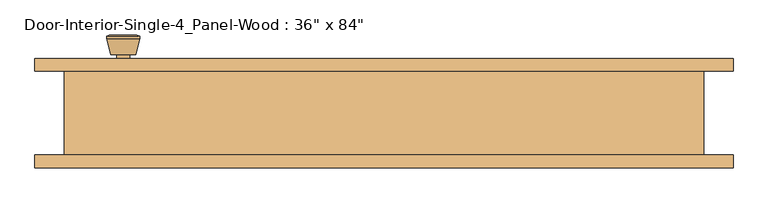
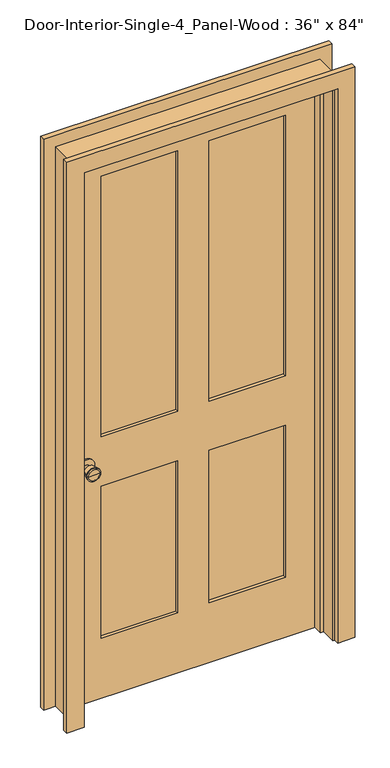
"""IFC4 building model written with IfcOpenShell, lengths in millimetres: door geometry."""

from ifc_helpers import new_model, si_unit, point, frame, frame_2d, origin, place, context, project, spatial, polyline, circle_curve, trimmed, segment, composite_curve, outline, extrude, faceted_brep, source, transform, mapped, element, save
from ifc_brep_helpers import plane_surface, cylinder_surface, revolved_surface, advanced_brep


def door_68a706ac(model_context):
    return source(origin(), model_context, "Body", "SolidModel", [
        advanced_brep(
        [(-393.7, 19.4, 914.4), (-383.7, 19.4, 914.4), (-403.7, 19.4, 914.4), (-373.2241324, -29.6, 914.4), (-393.7, -29.6, 914.4), (-414.1758676, -29.6, 914.4), (-368.7, -27.7721319, 914.4), (-418.7, -27.7721319, 914.4), (-368.7, -24.3084537, 914.4), (-418.7, -24.3084537, 914.4), (-375.063764, 0.4, 914.4), (-412.336236, 0.4, 914.4), (-383.7, 0.4, 914.4), (-403.7, 0.4, 914.4)],
        [
            (0, 1),
            (1, 2, circle_curve(frame((-393.7, 19.4, 914.4), z_axis=(0.0, 1.0, 0.0), x_axis=(-1.0, 0.0, 0.0)), 10.0)),
            (2, 0),
            (2, 1, circle_curve(frame((-393.7, 19.4, 914.4), z_axis=(0.0, 1.0, 0.0), x_axis=(-1.0, 0.0, 0.0)), 10.0)),
            (3, 4),
            (4, 5),
            (5, 3, circle_curve(frame((-393.7, -29.6, 914.4), z_axis=(0.0, -1.0, 0.0), x_axis=(-1.0, 0.0, 0.0)), 20.4758676)),
            (3, 5, circle_curve(frame((-393.7, -29.6, 914.4), z_axis=(0.0, -1.0, 0.0), x_axis=(-1.0, 0.0, 0.0)), 20.4758676)),
            (6, 3),
            (5, 7),
            (7, 6, circle_curve(frame((-393.7, -27.7721319, 914.4), z_axis=(0.0, -1.0, 0.0), x_axis=(-1.0, 0.0, 0.0)), 25.0)),
            (6, 7, circle_curve(frame((-393.7, -27.7721319, 914.4), z_axis=(0.0, -1.0, 0.0), x_axis=(-1.0, 0.0, 0.0)), 25.0)),
            (8, 6),
            (7, 9),
            (9, 8, circle_curve(frame((-393.7, -24.3084537, 914.4), z_axis=(0.0, -1.0, 0.0), x_axis=(-1.0, 0.0, 0.0)), 25.0)),
            (8, 9, circle_curve(frame((-393.7, -24.3084537, 914.4), z_axis=(0.0, -1.0, 0.0), x_axis=(-1.0, 0.0, 0.0)), 25.0)),
            (10, 8),
            (9, 11),
            (11, 10, circle_curve(frame((-393.7, 0.4, 914.4), z_axis=(0.0, -1.0, 0.0), x_axis=(-1.0, 0.0, 0.0)), 18.636236)),
            (10, 11, circle_curve(frame((-393.7, 0.4, 914.4), z_axis=(0.0, -1.0, 0.0), x_axis=(-1.0, 0.0, 0.0)), 18.636236)),
            (12, 10),
            (11, 13),
            (13, 12, circle_curve(frame((-393.7, 0.4, 914.4), z_axis=(0.0, -1.0, 0.0), x_axis=(-1.0, 0.0, 0.0)), 10.0)),
            (12, 13, circle_curve(frame((-393.7, 0.4, 914.4), z_axis=(0.0, -1.0, 0.0), x_axis=(-1.0, 0.0, 0.0)), 10.0)),
            (1, 12),
            (13, 2),
        ],
        [
            plane_surface(frame((-393.7, 19.4, 914.4), z_axis=(0.0, 1.0, 0.0), x_axis=(-1.0, 0.0, 0.0))),
            plane_surface(frame((-393.7, -29.6, 914.4), z_axis=(0.0, -1.0, 0.0), x_axis=(-1.0, 0.0, 0.0))),
            revolved_surface(polyline([(-414.1758676, -29.6, 914.4), (-418.7, -27.7721319, 914.4)]), (-393.7, 19.4, 914.4), (0.0, 1.0, 0.0)),
            cylinder_surface(frame((-393.7, 19.4, 914.4), z_axis=(0.0, 1.0, 0.0), x_axis=(-1.0, 0.0, 0.0)), 25.0),
            revolved_surface(polyline([(-418.7, -24.3084537, 914.4), (-412.336236, 0.4, 914.4)]), (-393.7, 19.4, 914.4), (0.0, 1.0, 0.0)),
            plane_surface(frame((-393.7, 0.4, 914.4), z_axis=(0.0, 1.0, 0.0), x_axis=(-1.0, 0.0, 0.0))),
            cylinder_surface(frame((-393.7, 19.4, 914.4), z_axis=(0.0, 1.0, 0.0), x_axis=(-1.0, 0.0, 0.0)), 10.0),
        ],
        [
            (0, [[1, 2, 3]]),
            (0, [[-3, 4, -1]]),
            (1, [[5, 6, 7]]),
            (1, [[-6, -5, 8]]),
            (2, [[9, -7, 10, 11]]),
            (2, [[-10, -8, -9, 12]]),
            (3, [[13, -11, 14, 15]]),
            (3, [[-14, -12, -13, 16]]),
            (4, [[17, -15, 18, 19]]),
            (4, [[-18, -16, -17, 20]]),
            (5, [[21, -19, 22, 23]]),
            (5, [[-22, -20, -21, 24]]),
            (6, [[25, -23, 26, -2]]),
            (6, [[-26, -24, -25, -4]]),
        ],
    ),
        extrude(outline(composite_curve([segment(trimmed(circle_curve(frame_2d((914.4, -393.7)), 30.0), [point((914.4, -423.7))], [point((914.4, -363.7))], False, "CARTESIAN"), True, "CONTINUOUS"), segment(trimmed(circle_curve(frame_2d((914.4, -393.7)), 30.0), [point((914.4, -363.7))], [point((914.4, -423.7))], False, "CARTESIAN"), True, "CONTINUOUS")], self_intersect=False)), frame((0.0, 19.4, 0.0), z_axis=(0.0, 1.0, 0.0), x_axis=(0.0, 0.0, 1.0)), (0.0, 0.0, 1.0), 6.0),
        advanced_brep(
        [(-393.7, 66.325, 914.4), (-403.7, 66.325, 914.4), (-383.7, 66.325, 914.4), (-373.2241324, 115.325, 914.4), (-414.1758676, 115.325, 914.4), (-393.7, 115.325, 914.4), (-368.7, 113.4971319, 914.4), (-418.7, 113.4971319, 914.4), (-368.7, 110.0334537, 914.4), (-418.7, 110.0334537, 914.4), (-375.063764, 85.325, 914.4), (-412.336236, 85.325, 914.4), (-383.7, 85.325, 914.4), (-403.7, 85.325, 914.4)],
        [
            (0, 1),
            (1, 2, circle_curve(frame((-393.7, 66.325, 914.4), z_axis=(0.0, -1.0, 0.0), x_axis=(-1.0, 0.0, 0.0)), 10.0)),
            (2, 0),
            (2, 1, circle_curve(frame((-393.7, 66.325, 914.4), z_axis=(0.0, -1.0, 0.0), x_axis=(-1.0, 0.0, 0.0)), 10.0)),
            (3, 4, circle_curve(frame((-393.7, 115.325, 914.4), z_axis=(0.0, 1.0, 0.0), x_axis=(-1.0, 0.0, 0.0)), 20.4758676)),
            (4, 5),
            (5, 3),
            (4, 3, circle_curve(frame((-393.7, 115.325, 914.4), z_axis=(0.0, 1.0, 0.0), x_axis=(-1.0, 0.0, 0.0)), 20.4758676)),
            (6, 7, circle_curve(frame((-393.7, 113.4971319, 914.4), z_axis=(0.0, 1.0, 0.0), x_axis=(-1.0, 0.0, 0.0)), 25.0)),
            (7, 4),
            (3, 6),
            (7, 6, circle_curve(frame((-393.7, 113.4971319, 914.4), z_axis=(0.0, 1.0, 0.0), x_axis=(-1.0, 0.0, 0.0)), 25.0)),
            (8, 9, circle_curve(frame((-393.7, 110.0334537, 914.4), z_axis=(0.0, 1.0, 0.0), x_axis=(-1.0, 0.0, 0.0)), 25.0)),
            (9, 7),
            (6, 8),
            (9, 8, circle_curve(frame((-393.7, 110.0334537, 914.4), z_axis=(0.0, 1.0, 0.0), x_axis=(-1.0, 0.0, 0.0)), 25.0)),
            (10, 11, circle_curve(frame((-393.7, 85.325, 914.4), z_axis=(0.0, 1.0, 0.0), x_axis=(-1.0, 0.0, 0.0)), 18.636236)),
            (11, 9),
            (8, 10),
            (11, 10, circle_curve(frame((-393.7, 85.325, 914.4), z_axis=(0.0, 1.0, 0.0), x_axis=(-1.0, 0.0, 0.0)), 18.636236)),
            (12, 13, circle_curve(frame((-393.7, 85.325, 914.4), z_axis=(0.0, 1.0, 0.0), x_axis=(-1.0, 0.0, 0.0)), 10.0)),
            (13, 11),
            (10, 12),
            (13, 12, circle_curve(frame((-393.7, 85.325, 914.4), z_axis=(0.0, 1.0, 0.0), x_axis=(-1.0, 0.0, 0.0)), 10.0)),
            (1, 13),
            (12, 2),
        ],
        [
            plane_surface(frame((-393.7, 66.325, 914.4), z_axis=(0.0, -1.0, 0.0), x_axis=(-1.0, 0.0, 0.0))),
            plane_surface(frame((-393.7, 115.325, 914.4), z_axis=(0.0, 1.0, 0.0), x_axis=(-1.0, 0.0, 0.0))),
            revolved_surface(polyline([(-414.1758676, 115.325, 914.4), (-418.7, 113.4971319, 914.4)]), (-393.7, 66.325, 914.4), (0.0, -1.0, 0.0)),
            cylinder_surface(frame((-393.7, 66.325, 914.4), z_axis=(0.0, -1.0, 0.0), x_axis=(-1.0, 0.0, 0.0)), 25.0),
            revolved_surface(polyline([(-418.7, 110.0334537, 914.4), (-412.336236, 85.325, 914.4)]), (-393.7, 66.325, 914.4), (0.0, -1.0, 0.0)),
            plane_surface(frame((-393.7, 85.325, 914.4), z_axis=(0.0, -1.0, 0.0), x_axis=(-1.0, 0.0, 0.0))),
            cylinder_surface(frame((-393.7, 66.325, 914.4), z_axis=(0.0, -1.0, 0.0), x_axis=(-1.0, 0.0, 0.0)), 10.0),
        ],
        [
            (0, [[1, 2, 3]]),
            (0, [[-3, 4, -1]]),
            (1, [[5, 6, 7]]),
            (1, [[8, -7, -6]]),
            (2, [[9, 10, -5, 11]]),
            (2, [[12, -11, -8, -10]]),
            (3, [[13, 14, -9, 15]]),
            (3, [[16, -15, -12, -14]]),
            (4, [[17, 18, -13, 19]]),
            (4, [[20, -19, -16, -18]]),
            (5, [[21, 22, -17, 23]]),
            (5, [[24, -23, -20, -22]]),
            (6, [[-2, 25, -21, 26]]),
            (6, [[-4, -26, -24, -25]]),
        ],
    ),
        extrude(outline(composite_curve([segment(trimmed(circle_curve(frame_2d((914.4, -393.7)), 30.0), [point((914.4, -423.7))], [point((914.4, -363.7))], False, "CARTESIAN"), True, "CONTINUOUS"), segment(trimmed(circle_curve(frame_2d((914.4, -393.7)), 30.0), [point((914.4, -363.7))], [point((914.4, -423.7))], False, "CARTESIAN"), True, "CONTINUOUS")], self_intersect=False)), frame((0.0, 60.325, 0.0), z_axis=(0.0, 1.0, 0.0), x_axis=(0.0, 0.0, 1.0)), (0.0, 0.0, 1.0), 6.0),
        faceted_brep([(482.6, 60.325, 0.0), (482.6, -66.675, 0.0), (457.2, -66.675, 0.0), (457.2, -9.525, 0.0), (444.5, -9.525, 0.0), (444.5, 25.4, 0.0), (457.2, 25.4, 0.0), (457.2, 60.325, 0.0), (482.6, 60.325, 2159.0), (482.6, -66.675, 2159.0), (-482.6, -66.675, 2159.0), (-482.6, -66.675, 0.0), (-457.2, -66.675, 0.0), (-457.2, -66.675, 2133.6), (457.2, -66.675, 2133.6), (457.2, -9.525, 2133.6), (-457.2, -9.525, 2133.6), (-457.2, -9.525, 0.0), (-444.5, -9.525, 0.0), (-444.5, -9.525, 2120.9), (444.5, -9.525, 2120.9), (444.5, 25.4, 2120.9), (-444.5, 25.4, 2120.9), (-444.5, 25.4, 0.0), (-457.2, 25.4, 0.0), (-457.2, 25.4, 2133.6), (457.2, 25.4, 2133.6), (457.2, 60.325, 2133.6), (-457.2, 60.325, 2133.6), (-457.2, 60.325, 0.0), (-482.6, 60.325, 0.0), (-482.6, 60.325, 2159.0)], [[[0, 1, 2, 3, 4, 5, 6, 7]], [[1, 0, 8, 9]], [[2, 1, 9, 10, 11, 12, 13, 14]], [[3, 2, 14, 15]], [[4, 3, 15, 16, 17, 18, 19, 20]], [[5, 4, 20, 21]], [[6, 5, 21, 22, 23, 24, 25, 26]], [[7, 6, 26, 27]], [[0, 7, 27, 28, 29, 30, 31, 8]], [[9, 8, 31, 10]], [[15, 14, 13, 16]], [[21, 20, 19, 22]], [[27, 26, 25, 28]], [[30, 29, 24, 23, 18, 17, 12, 11]], [[10, 31, 30, 11]], [[16, 13, 12, 17]], [[22, 19, 18, 23]], [[28, 25, 24, 29]]]),
        extrude(outline(polyline([(2133.6, -457.2), (0.0, -457.2), (0.0, 457.2), (2133.6, 457.2), (2133.6, -457.2)]), holes=[polyline([(2014.5375, 57.15), (2014.5375, 336.55), (1009.65, 336.55), (1009.65, 57.15), (2014.5375, 57.15)]), polyline([(1009.65, -57.15), (1009.65, -336.55), (2014.5375, -336.55), (2014.5375, -57.15), (1009.65, -57.15)]), polyline([(819.15, 57.15), (819.15, 336.55), (231.775, 336.55), (231.775, 57.15), (819.15, 57.15)]), polyline([(231.775, -57.15), (231.775, -336.55), (819.15, -336.55), (819.15, -57.15), (231.775, -57.15)])]), frame((0.0, 25.4, 0.0), z_axis=(0.0, 1.0, 0.0), x_axis=(0.0, 0.0, 1.0)), (0.0, 0.0, 1.0), 34.925),
        extrude(outline(polyline([(336.55, 37.0416667), (57.15, 37.0416667), (57.15, 48.6833333), (336.55, 48.6833333), (336.55, 37.0416667)])), frame((0.0, 0.0, 1009.65), z_axis=(0.0, 0.0, 1.0), x_axis=(1.0, 0.0, 0.0)), (0.0, 0.0, 1.0), 1004.8875),
        extrude(outline(polyline([(-57.15, 37.0416667), (-336.55, 37.0416667), (-336.55, 48.6833333), (-57.15, 48.6833333), (-57.15, 37.0416667)])), frame((0.0, 0.0, 1009.65), z_axis=(0.0, 0.0, 1.0), x_axis=(1.0, 0.0, 0.0)), (0.0, 0.0, 1.0), 1004.8875),
        extrude(outline(polyline([(336.55, 37.0416667), (57.15, 37.0416667), (57.15, 48.6833333), (336.55, 48.6833333), (336.55, 37.0416667)])), frame((0.0, 0.0, 231.775), z_axis=(0.0, 0.0, 1.0), x_axis=(1.0, 0.0, 0.0)), (0.0, 0.0, 1.0), 587.375),
        extrude(outline(polyline([(-57.15, 37.0416667), (-336.55, 37.0416667), (-336.55, 48.6833333), (-57.15, 48.6833333), (-57.15, 37.0416667)])), frame((0.0, 0.0, 231.775), z_axis=(0.0, 0.0, 1.0), x_axis=(1.0, 0.0, 0.0)), (0.0, 0.0, 1.0), 587.375),
        extrude(outline(polyline([(0.0, 463.55), (0.0, 527.05), (2203.45, 527.05), (2203.45, -527.05), (0.0, -527.05), (0.0, -463.55), (2139.95, -463.55), (2139.95, 463.55), (0.0, 463.55)])), frame((0.0, 60.325, 0.0), z_axis=(0.0, 1.0, 0.0), x_axis=(0.0, 0.0, 1.0)), (0.0, 0.0, 1.0), 19.05),
        extrude(outline(polyline([(0.0, 463.55), (0.0, 527.05), (2203.45, 527.05), (2203.45, -527.05), (0.0, -527.05), (0.0, -463.55), (2139.95, -463.55), (2139.95, 463.55), (0.0, 463.55)])), frame((0.0, -85.725, 0.0), z_axis=(0.0, 1.0, 0.0), x_axis=(0.0, 0.0, 1.0)), (0.0, 0.0, 1.0), 19.05),
    ])


if __name__ == "__main__":
    model = new_model("IFC4")
    model_context = context("Model", 3, world=origin())
    ifc_project = project(units=[si_unit("LENGTHUNIT", "METRE", prefix="MILLI")], contexts=[model_context])
    site = spatial("IfcSite", under=ifc_project)
    building = spatial("IfcBuilding", under=site)
    placement = place(None, origin())
    door_shape = door_68a706ac(model_context)
    element("IfcDoor", 1, ObjectType="Door-Interior-Single-4_Panel-Wood : 36\" x 84\"", at=placement, inside=building, context=model_context, shape_type="MappedRepresentation", body=[
        mapped(door_shape, transform((0.0, 0.0, 0.0), x_axis=(1.0, 0.0, 0.0), y_axis=(0.0, 1.0, 0.0), z_axis=(0.0, 0.0, 1.0))),
    ])
    save(model, "model.ifc")

# Revit data of these elements
# Type "Door-Interior-Single-4_Panel-Wood : 36\" x 84\""
#   Type Mark = "10"
#   Assembly Code = "C1020300"
#   Analytic Construction = "Wooden"
#   Top Rail = 0' - 4 11/16"
#   Thickness = 0' - 1 3/8"
#   Thermal Resistance (R) = 2.5876 (h·ft²·°F)/BTU
#   Swing Angle [instance default] = 90.00°
#   Stiles = 0' - 4 3/4"
#   Rough Width = 3' - 2"
#   Rough Height = 7' - 1"
#   Mullion = 0' - 4 1/2"
#   Lock Rail = 0' - 7 1/2"
#   Height = 7' - 0"
#   Width = 3' - 0"
#   Heat Transfer Coefficient (U) = 0.3865 BTU/(h·ft²·°F)
#   Bottom Rail = 0' - 9 1/8"
#   Trim Material = Cherry
#   Panel Material = Cherry
#   Frame Material = Cherry
#   Door Handle Material = Aluminum
#   Visual Light Transmittance = 0
#   Solar Heat Gain Coefficient = 0
#   Wall Closure = (empty or 0)
#   Function = (empty or 0)
# Element 1 (IfcDoor, "Door-Interior-Single-4_Panel-Wood : 36\" x 84\"")
#   Materials on its faces: "Cherry", "Aluminum"
# Materials
#   "Cherry": class "Wood", colour RGB 226 177 128, transparency 0, Description = "Prunus Serotina", Cost = 0
#   "Aluminum": class "Metal", colour RGB 247 247 247, transparency 0, Description = "Aluminum 6061", Cost = 0
